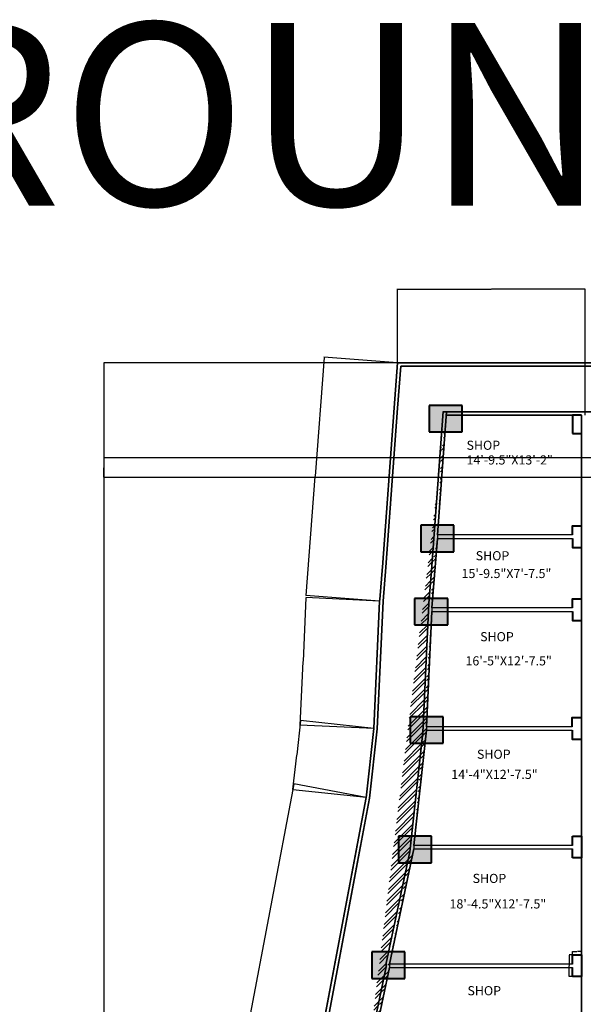
# Model space of a CAD drawing. Units: inches. Extents: x 1563 to 5866, y -225 to 2207.
# Tile 2 of 3: x 2883 to 3624, y 913 to 2207. Entities that reach past the tile are written whole.
import ezdxf

# ---------------------------------------------------------------- set-up
doc = ezdxf.new("R2010")
doc.units = ezdxf.units.IN
for name, color, linetype, lineweight in [('A-ANNO-DIMS', 2, 'Continuous', 18), ('A-ANNO-TEXT', 7, 'Continuous', 25), ('A-AREA-IDEN', 7, 'Continuous', 18), ('A-COLS', 1, 'Continuous', 40), ('A-WALL', 7, 'Continuous', 35), ('A-WALL-INTR', 7, 'Continuous', 30), ('A-WALL-PATT', 8, 'Continuous', 13), ('C-PROP', 2, 'Continuous', 35)]:
    doc.layers.add(name, color=color, linetype=linetype, lineweight=lineweight)
doc.styles.get("Standard").update_dxf_attribs({"font": 'arial.ttf'})
doc.dimstyles.get("Standard").update_dxf_attribs({"dimtxt": 0.18, "dimasz": 0.18, "dimexe": 0.18, "dimexo": 0.0625, "dimgap": 0.09, "dimtad": 0, "dimtih": 1, "dimtoh": 1, "dimdec": 4, "dimzin": 0, "dimdsep": 46, "dimtxsty": 'Standard', "dimcen": 0.09, "dimadec": 0, "dimazin": 0, "dimtfac": 1, "dimtdec": 4, "dimtofl": 0, "dimtmove": 0, "dimatfit": 3, "dimfxl": 1, "dimtolj": 1, "dimtzin": 0, "dimarcsym": 0})

# ---------------------------------------------------------------- blocks, each defined once
blk = doc.blocks.new('COL-RECT-FILLED')
h = blk.add_hatch(color=256)
h.dxf.hatch_style = 1
h.paths.add_polyline_path([(0, 34.9), (0, 0), (43.4, 0), (43.4, 34.9)])
for p, q in [((43.4, 34.9), (0, 34.9)), ((0, 34.9), (0, 0)), ((43.4, 0), (43.4, 34.9)), ((0, 0), (43.4, 0))]:
    blk.add_line(p, q)
blk = doc.blocks.new('PIER-SHOP-RETURN-1')
for p, q in [((0, 16.5), (0, 28.5)), ((0, 28.5), (12, 28.5)), ((12, 28.5), (12, 16.5)), ((12, 16.5), (12, 12)), ((0, 0), (0, 12)), ((12, 12), (12, 0)), ((12, 0), (0, 0))]:
    blk.add_line(p, q)
blk = doc.blocks.new('*D12')
at = {"layer": 'A-ANNO-DIMS', "color": 0, "lineweight": -2, "transparency": 16777216}
for p, q in [((3609.4, 978), (3605, 978)), ((3605.2, 977.8), (3605.2, 963.9)), ((3605.2, 949.7), (3605.2, 963.6)), ((3609.4, 949.5), (3605, 949.5))]:
    blk.add_line(p, q, dxfattribs=at)
at = {"layer": 'A-ANNO-DIMS', "color": 0, "transparency": 16777216}
for points in [[(3605.2, 977.8), (3605.2, 977.8), (3605.2, 978)], [(3605.2, 949.7), (3605.2, 949.7), (3605.2, 949.5)]]:
    blk.add_solid(points, dxfattribs=at)
at = {"layer": 'Defpoints', "color": 0, "transparency": 16777216}
for p in [(3605.2, 978), (3609.5, 978), (3609.5, 949.5)]:
    blk.add_point(p, dxfattribs=at)
at = {"layer": 'A-ANNO-DIMS', "color": 0, "transparency": 16777216, "insert": (3605.2, 963.8), "char_height": 0.18, "attachment_point": 5}
blk.add_mtext('\\A1;RETURN PIER 1 29 TYP.', dxfattribs=at)
blk = doc.blocks.new('*D13')
at = {"layer": 'A-ANNO-DIMS', "color": 0, "lineweight": -2, "transparency": 16777216}
for p, q in [((3609.5, 978.1), (3609.5, 982.5)), ((3609.7, 982.3), (3615, 982.3)), ((3621.3, 982.3), (3616, 982.3)), ((3621.5, 978.1), (3621.5, 982.5))]:
    blk.add_line(p, q, dxfattribs=at)
at = {"layer": 'A-ANNO-DIMS', "color": 0, "transparency": 16777216}
for points in [[(3609.7, 982.3), (3609.7, 982.3), (3609.5, 982.3)], [(3621.3, 982.3), (3621.3, 982.3), (3621.5, 982.3)]]:
    blk.add_solid(points, dxfattribs=at)
at = {"layer": 'Defpoints', "color": 0, "transparency": 16777216}
for p in [(3609.5, 978), (3621.5, 982.3), (3621.5, 978)]:
    blk.add_point(p, dxfattribs=at)
at = {"layer": 'A-ANNO-DIMS', "color": 0, "transparency": 16777216, "insert": (3615.5, 982.3), "char_height": 0.18, "attachment_point": 5}
blk.add_mtext('\\A1;12 TYP.', dxfattribs=at)
blk = doc.blocks.new('*D19')
at = {"layer": 'A-ANNO-DIMS', "color": 0, "lineweight": -2, "transparency": 16777216}
for p, q in [((3379.5, 1756.3), (2993.3, 1756.3)), ((2993.5, 1756.1), (2993.5, 814.2)), ((2993.5, -128), (2993.5, 813.9)), ((3090.3, -128.2), (2993.3, -128.2))]:
    blk.add_line(p, q, dxfattribs=at)
at = {"layer": 'A-ANNO-DIMS', "color": 0, "transparency": 16777216}
for points in [[(2993.4, 1756.1), (2993.5, 1756.1), (2993.5, 1756.3)], [(2993.4, -128), (2993.5, -128), (2993.5, -128.2)]]:
    blk.add_solid(points, dxfattribs=at)
at = {"layer": 'Defpoints', "color": 0, "transparency": 16777216}
for p in [(2993.5, 1756.3), (3379.6, 1756.3), (3090.4, -128.2)]:
    blk.add_point(p, dxfattribs=at)
at = {"layer": 'A-ANNO-DIMS', "color": 0, "transparency": 16777216, "insert": (2993.5, 814), "char_height": 0.18, "attachment_point": 5}
blk.add_mtext('\\A1;1884.5', dxfattribs=at)
blk = doc.blocks.new('*D20')
at = {"layer": 'A-ANNO-DIMS', "color": 0, "lineweight": -2, "transparency": 16777216}
for p, q in [((3379.6, 1756.4), (3379.6, 1853.4)), ((3379.8, 1853.2), (3502.4, 1853.2)), ((3625.8, 1853.2), (3503.2, 1853.2)), ((3626, 1687.4), (3626, 1853.4))]:
    blk.add_line(p, q, dxfattribs=at)
at = {"layer": 'A-ANNO-DIMS', "color": 0, "transparency": 16777216}
for points in [[(3379.8, 1853.2), (3379.8, 1853.2), (3379.6, 1853.2)], [(3625.8, 1853.2), (3625.8, 1853.2), (3626, 1853.2)]]:
    blk.add_solid(points, dxfattribs=at)
at = {"layer": 'Defpoints', "color": 0, "transparency": 16777216}
for p in [(3626, 1853.2), (3379.6, 1756.3), (3626, 1687.3)]:
    blk.add_point(p, dxfattribs=at)
at = {"layer": 'A-ANNO-DIMS', "color": 0, "transparency": 16777216, "insert": (3502.8, 1853.2), "char_height": 0.18, "attachment_point": 5}
blk.add_mtext('\\A1;246.4', dxfattribs=at)
blk = doc.blocks.new('*D35')
at = {"layer": 'A-ANNO-DIMS', "color": 0, "lineweight": -2, "transparency": 16777216}
for p, q in [((3243.1, 1202.5), (3119.2, 546.4)), ((3338.3, 1184.7), (3243, 1202.7)), ((2995.2, -110.1), (3119.1, 546)), ((3090.3, -128.2), (2995, -110.2))]:
    blk.add_line(p, q, dxfattribs=at)
at = {"layer": 'A-ANNO-DIMS', "color": 0, "transparency": 16777216}
for points in [[(3243.1, 1202.5), (3243.2, 1202.5), (3243.2, 1202.7)], [(2995.2, -110.1), (2995.2, -110.1), (2995.2, -110.2)]]:
    blk.add_solid(points, dxfattribs=at)
at = {"layer": 'Defpoints', "color": 0, "transparency": 16777216}
for p in [(3243.2, 1202.7), (3338.4, 1184.7), (3090.4, -128.2)]:
    blk.add_point(p, dxfattribs=at)
at = {"layer": 'A-ANNO-DIMS', "color": 0, "transparency": 16777216, "insert": (3119.2, 546.2), "char_height": 0.18, "attachment_point": 5}
blk.add_mtext('\\A1;1336', dxfattribs=at)
blk = doc.blocks.new('*D36')
at = {"layer": 'A-ANNO-DIMS', "color": 0, "lineweight": -2, "transparency": 16777216}
for p, q in [((3251.9, 1285.8), (3247, 1240.8)), ((3348.2, 1275.5), (3251.8, 1286)), ((3242.1, 1195.4), (3247, 1240.4)), ((3338.3, 1184.7), (3241.9, 1195.2))]:
    blk.add_line(p, q, dxfattribs=at)
at = {"layer": 'A-ANNO-DIMS', "color": 0, "transparency": 16777216}
for points in [[(3251.9, 1285.9), (3252, 1285.8), (3252, 1286)], [(3242.1, 1195.4), (3242.1, 1195.3), (3242.1, 1195.2)]]:
    blk.add_solid(points, dxfattribs=at)
at = {"layer": 'Defpoints', "color": 0, "transparency": 16777216}
for p in [(3252, 1286), (3348.3, 1275.5), (3338.4, 1184.7)]:
    blk.add_point(p, dxfattribs=at)
at = {"layer": 'A-ANNO-DIMS', "color": 0, "transparency": 16777216, "insert": (3247, 1240.6), "char_height": 0.18, "attachment_point": 5}
blk.add_mtext('\\A1;91.4', dxfattribs=at)
blk = doc.blocks.new('*D37')
at = {"layer": 'A-ANNO-DIMS', "color": 0, "lineweight": -2, "transparency": 16777216}
for p, q in [((3259.2, 1447.4), (3255.4, 1364)), ((3356, 1443.1), (3259.1, 1447.6)), ((3251.5, 1280.2), (3255.4, 1363.6)), ((3348.2, 1275.5), (3251.3, 1280))]:
    blk.add_line(p, q, dxfattribs=at)
at = {"layer": 'A-ANNO-DIMS', "color": 0, "transparency": 16777216}
for points in [[(3259.2, 1447.4), (3259.3, 1447.4), (3259.2, 1447.6)], [(3251.5, 1280.2), (3251.5, 1280.2), (3251.5, 1280)]]:
    blk.add_solid(points, dxfattribs=at)
at = {"layer": 'Defpoints', "color": 0, "transparency": 16777216}
for p in [(3259.2, 1447.6), (3356, 1443.1), (3348.3, 1275.5)]:
    blk.add_point(p, dxfattribs=at)
at = {"layer": 'A-ANNO-DIMS', "color": 0, "transparency": 16777216, "insert": (3255.4, 1363.8), "char_height": 0.18, "attachment_point": 5}
blk.add_mtext('\\A1;167.74', dxfattribs=at)
blk = doc.blocks.new('*D38')
at = {"layer": 'A-ANNO-DIMS', "color": 0, "lineweight": -2, "transparency": 16777216}
for p, q in [((3282.9, 1763.4), (3271.2, 1607.1)), ((3379.5, 1756.3), (3282.8, 1763.6)), ((3259.4, 1450.5), (3271.2, 1606.8)), ((3356, 1443.1), (3259.2, 1450.4))]:
    blk.add_line(p, q, dxfattribs=at)
at = {"layer": 'A-ANNO-DIMS', "color": 0, "transparency": 16777216}
for points in [[(3282.9, 1763.4), (3283, 1763.4), (3282.9, 1763.6)], [(3259.4, 1450.5), (3259.4, 1450.5), (3259.4, 1450.4)]]:
    blk.add_solid(points, dxfattribs=at)
at = {"layer": 'Defpoints', "color": 0, "transparency": 16777216}
for p in [(3282.9, 1763.6), (3379.6, 1756.3), (3356, 1443.1)]:
    blk.add_point(p, dxfattribs=at)
at = {"layer": 'A-ANNO-DIMS', "color": 0, "transparency": 16777216, "insert": (3271.2, 1607), "char_height": 0.18, "attachment_point": 5}
blk.add_mtext('\\A1;314.1', dxfattribs=at)
blk = doc.blocks.new('*D44')
at = {"layer": 'A-ANNO-DIMS', "color": 0, "lineweight": -2, "transparency": 16777216}
for p, q in [((3845.4, 1631.6), (2993.3, 1631.6)), ((2993.5, 1631.4), (2993.5, 1618.8)), ((2993.5, 1605.8), (2993.5, 1618.4)), ((3845.4, 1605.6), (2993.3, 1605.6))]:
    blk.add_line(p, q, dxfattribs=at)
at = {"layer": 'A-ANNO-DIMS', "color": 0, "transparency": 16777216}
for points in [[(2993.4, 1631.4), (2993.5, 1631.4), (2993.5, 1631.6)], [(2993.4, 1605.8), (2993.5, 1605.8), (2993.5, 1605.6)]]:
    blk.add_solid(points, dxfattribs=at)
at = {"layer": 'Defpoints', "color": 0, "transparency": 16777216}
for p in [(2993.5, 1631.6), (3845.5, 1631.6), (3845.5, 1605.6)]:
    blk.add_point(p, dxfattribs=at)
at = {"layer": 'A-ANNO-DIMS', "color": 0, "transparency": 16777216, "insert": (2993.5, 1618.6), "char_height": 0.18, "attachment_point": 5}
blk.add_mtext('\\A1;25.95', dxfattribs=at)

msp = doc.modelspace()

# ---------------------------------------------------------------- hatches: boundary and pattern name
at = {"layer": 'A-WALL-PATT'}
h = msp.add_hatch(dxfattribs=at)
h.set_pattern_fill('ANSI32', color=256)
edge = h.paths.add_edge_path()
edge.add_line((3443.9794, 1691.8133), (3431.9794, 1530.0177))
edge.add_line((3439.4917, 1692.1461), (3423.9855, 1483.0764))
edge.add_line((3431.9794, 1525.5177), (3424.4794, 1434.0177))
edge.add_line((3423.9855, 1483.0764), (3420.4644, 1440.1194))
edge.add_line((3420.4644, 1440.1194), (3412.6295, 1270.5497))
edge.add_line((3424.4794, 1429.5177), (3417.4794, 1278.0177))
edge.add_line((3417.4794, 1273.5177), (3400.9794, 1122.0177))
edge.add_line((3412.6295, 1270.5497), (3395.5183, 1113.4377))
edge.add_line((3400.9794, 1117.5177), (3368.9794, 966.0177))
edge.add_line((3395.5183, 1113.4377), (3364.5765, 966.9477))
edge.add_line((3368.9794, 966.0177), (3368.9794, 961.5177))
edge.add_line((3364.5765, 966.9477), (3364.5765, 962.4477))
edge.add_line((3368.9794, 961.5177), (3336.9794, 810.0177))
edge.add_line((3364.5765, 962.4477), (3340.6094, 848.9784))
edge.add_line((3340.6094, 848.9784), (3301.0547, 639.5806))
edge.add_line((3336.9794, 810.0177), (3336.9794, 805.5177))
edge.add_line((3336.9794, 805.5177), (3304.9794, 636.1136))
edge.add_line((3301.0547, 639.5806), (3285.4229, 427.6136))
edge.add_line((3304.9794, 636.1136), (3304.9794, 631.6136))
edge.add_line((3304.9794, 631.6136), (3289.9351, 427.6136))

# ---------------------------------------------------------------- linework, layer by layer
at = {"layer": 'A-COLS'}
for p, q in [((3621.4794, 1687.3133), (3609.4794, 1687.3133)), ((3609.4794, 1687.3133), (3609.4794, 1675.3133)), ((3609.4794, 1675.3133), (3609.4794, 1663.3133)), ((3609.4794, 1663.3133), (3621.4794, 1663.3133))]:
    msp.add_line(p, q, dxfattribs=at)
for points in [[(3609.3934, 1530.0177), (3609.3934, 1542.0498), (3621.4794, 1542.0498)], [(3609.3934, 1525.5177), (3609.3934, 1513.5498), (3621.4794, 1513.5498)], [(3609.4794, 1434.0177), (3609.4794, 1446.0177), (3621.4794, 1446.0177)], [(3609.4794, 1429.5177), (3609.4794, 1417.5177), (3621.4794, 1417.5177)], [(3609.1749, 1278.0177), (3609.1749, 1290.1616), (3621.4794, 1290.1616)], [(3609.1749, 1273.5177), (3609.1749, 1261.6616), (3621.4794, 1261.6616)]]:
    msp.add_lwpolyline(points, dxfattribs=at)
at = {"layer": 'A-WALL'}
for p, q in [((3439.4917, 1692.1461), (3423.9855, 1483.0764)), ((3443.9794, 1691.8133), (3431.9794, 1530.0177)), ((3443.9794, 1691.8133), (3439.4794, 1691.8133)), ((3621.4794, 1687.3133), (3443.6456, 1687.3133)), ((3621.4794, 1691.8133), (3443.9794, 1691.8133)), ((3621.4794, 1691.8133), (3727.4794, 1691.8133)), ((3621.4794, 1687.3133), (3621.4794, 495.9392)), ((3431.9794, 1525.5177), (3424.4794, 1434.0177)), ((3423.9855, 1483.0764), (3420.4644, 1440.1194)), ((3420.4644, 1440.1194), (3412.6295, 1270.5497)), ((3424.4794, 1429.5177), (3417.4794, 1278.0177)), ((3621.4794, 1369.5177), (3621.4794, 1218.0177)), ((3412.6295, 1270.5497), (3395.5183, 1113.4377)), ((3417.4794, 1273.5177), (3400.9794, 1122.0177)), ((3395.5183, 1113.4377), (3364.5765, 966.9477)), ((3400.9794, 1117.5177), (3368.9794, 966.0177)), ((3368.9794, 961.5177), (3336.9794, 810.0177)), ((3364.5765, 962.4477), (3340.6094, 848.9784)), ((3364.5765, 966.9477), (3364.5765, 962.4477))]:
    msp.add_line(p, q, dxfattribs=at)
at = {"layer": 'A-WALL-INTR'}
for p, q in [((3609.3934, 1530.0177), (3431.9794, 1530.0177)), ((3431.9794, 1530.0177), (3431.9794, 1525.5177)), ((3431.9794, 1525.5177), (3609.3934, 1525.5177)), ((3609.4794, 1434.0177), (3424.4794, 1434.0177)), ((3424.4794, 1434.0177), (3424.4794, 1429.5177)), ((3424.4794, 1429.5177), (3609.4794, 1429.5177)), ((3609.1749, 1278.0177), (3417.4794, 1278.0177)), ((3417.4794, 1278.0177), (3417.4794, 1273.5177)), ((3417.4794, 1273.5177), (3609.1749, 1273.5177)), ((3609.4794, 1122.0177), (3400.9794, 1122.0177)), ((3400.9794, 1122.0177), (3400.9794, 1117.5177)), ((3400.9794, 1117.5177), (3609.4794, 1117.5177)), ((3609.4794, 966.0177), (3368.9794, 966.0177)), ((3368.9794, 966.0177), (3368.9794, 961.5177)), ((3368.9794, 961.5177), (3609.4794, 961.5177))]:
    msp.add_line(p, q, dxfattribs=at)
at = {"layer": 'C-PROP'}
for p, q in [((3375.1684, 1696.9168), (3379.5737, 1756.3133)), ((3383.7523, 1756.3133), (3379.5737, 1756.3133)), ((3379.6561, 1696.584), (3383.7523, 1751.8133)), ((3383.7523, 1751.8133), (3383.7523, 1751.8133)), ((3375.1684, 1696.9168), (3359.6622, 1487.8471)), ((3379.6561, 1696.584), (3364.1498, 1487.5142)), ((3359.7011, 1488.3456), (3356.18, 1445.3886)), ((3364.1498, 1487.5142), (3360.5284, 1442.8887)), ((3356.0332, 1443.0964), (3348.291, 1275.5348)), ((3360.5284, 1442.8887), (3352.7798, 1275.187)), ((3356.18, 1445.3886), (3356.0332, 1443.0964)), ((3348.291, 1275.5348), (3338.396, 1184.6804)), ((3352.7798, 1275.187), (3342.8696, 1184.1932)), ((3338.4478, 1185.0285), (3237.6755, 651.5527)), ((3342.8696, 1184.1932), (3242.0973, 650.7174)), ((3330.967, 1121.1824), (3096.721, -118.8872))]:
    msp.add_line(p, q, dxfattribs=at)
for points in [[(3383.7523, 1756.3133), (3621.4794, 1756.3133), (4062.0619, 1756.3133)], [(3383.7523, 1751.8133), (3621.4794, 1751.8133), (4057.5619, 1751.8133)], [(3326.5452, 1122.0177), (3090.3766, -128.2295), (3550.7842, 163.2371), (3788.3855, 293.8419), (3941.0013, 377.7319), (4062.0619, 444.2765)]]:
    msp.add_lwpolyline(points, dxfattribs=at)

# ---------------------------------------------------------------- block references
at = {"layer": 'A-COLS'}
for name, p in [('COL-RECT-FILLED', (3420.9218, 1665.4467)), ('COL-RECT-FILLED', (3410.1845, 1507.9662)), ('COL-RECT-FILLED', (3402.0376, 1411.7639)), ('COL-RECT-FILLED', (3396.1126, 1256.1201)), ('COL-RECT-FILLED', (3380.9354, 1099.0468)), ('PIER-SHOP-RETURN-1', (3609.4794, 1105.5177)), ('COL-RECT-FILLED', (3345.7554, 947.1559)), ('PIER-SHOP-RETURN-1', (3609.4794, 949.5177))]:
    msp.add_blockref(name, p, dxfattribs=at)

# ---------------------------------------------------------------- texts
at = {"layer": 'A-ANNO-TEXT'}
msp.add_text('SHOP GROUND FLOOR PLAN', height=240, dxfattribs=at).set_placement((1547.6082, 1963.0298))
at = {"layer": 'A-AREA-IDEN'}
for s, p in [('SHOP', (3470.2203, 1641.9008)), ('14\'-9.5"X13\'-2"', (3470.2203, 1622.6239)), ('SHOP', (3482.2727, 1496.7027)), ('15\'-9.5"X7\'-7.5"', (3463.675, 1473.3776)), ('SHOP', (3488.0946, 1390.3304)), ('16\'-5"X12\'-7.5"', (3468.8586, 1358.5335)), ('SHOP', (3483.9448, 1235.7901)), ('14\'-4"X12\'-7.5"', (3450.1882, 1209.2923)), ('SHOP', (3478.2332, 1072.5746)), ('18\'-4.5"X12\'-7.5"', (3447.8544, 1039.0641)), ('SHOP', (3471.4145, 924.9711))]:
    msp.add_text(s, height=12, dxfattribs=at).set_placement(p)

# ---------------------------------------------------------------- dimensions: what is measured, and where the dimension line sits
at = {"layer": 'A-ANNO-DIMS'}
dim = msp.add_linear_dim(base=(3625.9794, 1853.2133), p1=(3379.5737, 1756.3133), p2=(3625.9794, 1687.3133), dimstyle='Standard', override={"dimdec": 1, "dimlfac": 1, "dimrnd": 0, "dimzin": 0, "dimdsep": 46, "dimlunit": 2}, dxfattribs=at)
dim.commit()
dim.dimension.update_dxf_attribs({"geometry": '*D20', "text_midpoint": (3502.7765, 1853.2133)})
for base, p1, p2, angle, override, picture, middle in [((3282.9462, 1763.5755), (3356.0332, 1443.0964), (3379.5737, 1756.3133), 85.7018887, {"dimdec": 1, "dimlfac": 1, "dimrnd": 0, "dimzin": 0, "dimdsep": 46, "dimlunit": 2}, '*D38', (3271.1759, 1606.9671)), ((2993.4766, 1756.3133), (3090.3766, -128.2295), (3379.5737, 1756.3133), 90, {"dimdec": 1, "dimlfac": 1, "dimrnd": 0, "dimzin": 0, "dimdsep": 46, "dimlunit": 2}, '*D19', (2993.4766, 814.0419)), ((2993.4766, 1631.5836), (3845.4794, 1605.6311), (3845.4794, 1631.5836), 90, {"dimdec": 2, "dimlfac": 1, "dimrnd": 0, "dimzin": 0, "dimdsep": 46, "dimlunit": 2}, '*D44', (2993.4766, 1618.6073)), ((3259.2364, 1447.5688), (3348.291, 1275.5348), (3356.0332, 1443.0964), 87.3545517, {"dimdec": 2, "dimlfac": 1, "dimrnd": 0, "dimzin": 0, "dimdsep": 46, "dimlunit": 2}, '*D37', (3255.3654, 1363.788)), ((3251.9607, 1286.0262), (3338.396, 1184.6804), (3348.291, 1275.5348), 83.7843641, {"dimdec": 1, "dimlfac": 1, "dimrnd": 0, "dimzin": 0, "dimdsep": 46, "dimlunit": 2}, '*D36', (3247.0132, 1240.599)), ((3243.1801, 1202.6675), (3090.3766, -128.2295), (3338.396, 1184.6804), 79.3024241, {"dimdec": 0, "dimlfac": 1, "dimrnd": 0, "dimzin": 0, "dimdsep": 46, "dimlunit": 2}, '*D35', (3119.1704, 546.2125))]:
    dim = msp.add_linear_dim(base=base, p1=p1, p2=p2, angle=angle, dimstyle='Standard', override=override, dxfattribs=at)
    dim.commit()
    dim.dimension.update_dxf_attribs({"geometry": picture, "text_midpoint": middle})
dim = msp.add_linear_dim(base=(3605.2043818998, 978.0176943851), p1=(3609.4793818998, 949.5176943851), p2=(3609.4793818998, 978.0176943851), angle=90, text='RETURN PIER 1 <> TYP.', dimstyle='Standard', override={"dimdec": 0, "dimlfac": 1, "dimrnd": 0, "dimzin": 0, "dimdsep": 46, "dimlunit": 2}, dxfattribs=at)
dim.commit()
dim.dimension.update_dxf_attribs({"geometry": '*D12', "text_midpoint": (3605.2043818998, 963.7676943851)})
dim = msp.add_linear_dim(base=(3621.4794, 982.2927), p1=(3609.4794, 978.0177), p2=(3621.4794, 978.0177), text='<> TYP.', dimstyle='Standard', override={"dimdec": 0, "dimlfac": 1, "dimrnd": 0, "dimzin": 0, "dimdsep": 46, "dimlunit": 2}, dxfattribs=at)
dim.commit()
dim.dimension.update_dxf_attribs({"geometry": '*D13', "text_midpoint": (3615.4794, 982.2927)})

doc.saveas('drawing.dxf')
